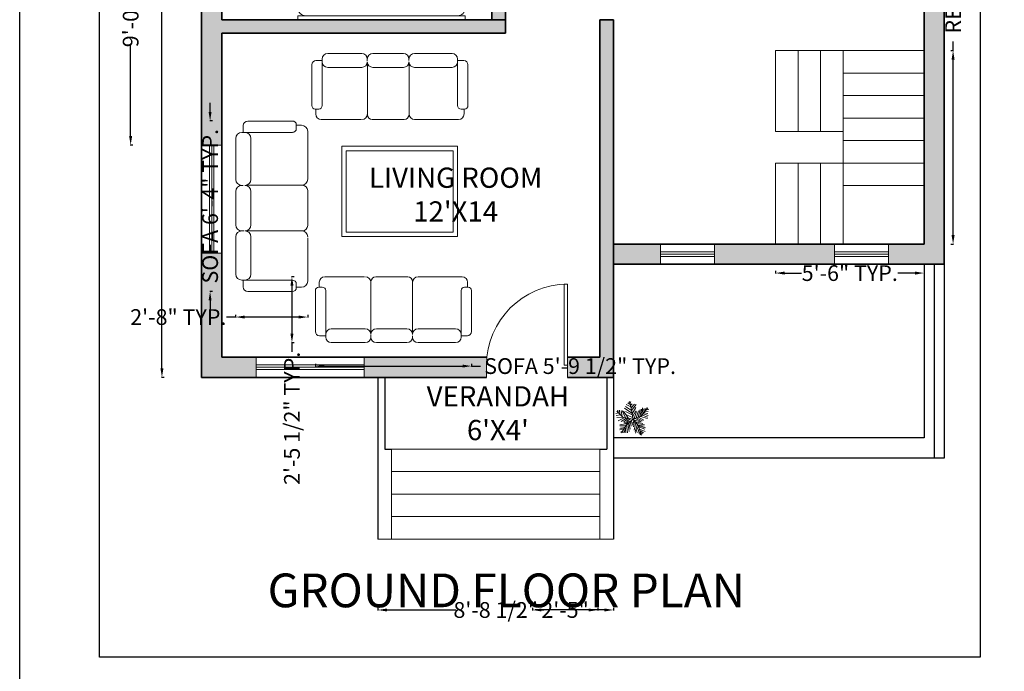
# Model space of a CAD drawing. Units: inches. Extents: x -80 to 1461, y -1239 to 153.
# Tile 2 of 6: x -80 to 358, y -562 to -273. Entities that reach past the tile are written whole.
import ezdxf

# ---------------------------------------------------------------- set-up
doc = ezdxf.new("R2010")
doc.units = ezdxf.units.IN
doc.header["$MEASUREMENT"] = 0
for name, color, linetype, lineweight in [('A-ANNO-DIMS', 2, 'Continuous', 18), ('A-ANNO-TEXT', 7, 'Continuous', 18), ('A-ANNO-TTLB', 7, 'Continuous', 25), ('A-AREA-IDEN', 7, 'Continuous', 18), ('A-FLOR', 7, 'Continuous', 25), ('A-FLOR-STRS', 7, 'Continuous', 20), ('A-FURN', 8, 'Continuous', 18), ('A-GLAZ', 4, 'Continuous', 18), ('A-WALL', 7, 'Continuous', 35), ('A-WALL-PATT', 8, 'Continuous', 13), ('DOOR', 32, 'Continuous', 18), ('TREE', 92, 'Continuous', 13)]:
    doc.layers.add(name, color=color, linetype=linetype, lineweight=lineweight)
doc.styles.get("Standard").update_dxf_attribs({"font": 'arial.ttf'})
doc.dimstyles.get("Standard").update_dxf_attribs({"dimtxt": 7, "dimasz": 4, "dimexe": 0.18, "dimexo": 0.0625, "dimgap": 0.09, "dimtad": 0, "dimdec": 0, "dimzin": 0, "dimdsep": 46, "dimlunit": 3, "dimtxsty": 'Standard', "dimcen": 0.09, "dimadec": 0, "dimazin": 0, "dimtfac": 1, "dimtdec": 0, "dimtofl": 0, "dimtmove": 0, "dimatfit": 3, "dimfxl": 1, "dimfxlon": 1, "dimtolj": 1, "dimtzin": 0, "dimarcsym": 0})

# ---------------------------------------------------------------- blocks, each defined once
blk = doc.blocks.new('*U2')
for p, q in [((0, 0), (0, -6)), ((40, 0), (40, -6))]:
    blk.add_line(p, q)
blk.add_lwpolyline([(0, 0), (0, 40), (1.75, 40), (1.75, 0)], close=True)
blk.add_arc((0, 0), 40, 0, 90)
blk = doc.blocks.new('A$C164346CA')
for p, q in [((0, 2.035), (0, 2)), ((1.5, 2.035), (0, 2.035)), ((1.5, 2), (1.5, 2.035)), ((1.5, 2), (0, 2)), ((0, 1.93), (0, 0.07)), ((0.0919, 1.8624), (0.0919, 1.6069)), ((0.6731, 1.9024), (0.1319, 1.9024)), ((0.7131, 1.6069), (0.7131, 1.8624)), ((0.7828, 1.8624), (0.7828, 1.6069)), ((1.364, 1.9024), (0.8228, 1.9024)), ((1.404, 1.6069), (1.404, 1.8624)), ((1.5, 0.07), (1.5, 1.93)), ((0.1319, 1.5669), (0.6731, 1.5669)), ((0.8228, 1.5669), (1.364, 1.5669)), ((0.8395, 1.4761), (0, 1.4761)), ((0.8395, 1.4761), (1.2448, 1.12)), ((1.5, 1.2611), (0.8395, 1.4761)), ((1.3077, 1.1175), (1.5, 1.2611)), ((0.07, 0), (1.43, 0))]:
    blk.add_line(p, q)
for centre, radius, start, end in [((0.07, 1.93), 0.07, 90, 180), ((1.43, 1.93), 0.07, 0, 90), ((0.1319, 1.8624), 0.04, 90, 180), ((0.6731, 1.8624), 0.04, 0, 90), ((0.8228, 1.8624), 0.04, 90, 180), ((1.364, 1.8624), 0.04, 0, 90), ((0.1319, 1.6069), 0.04, 180, 270), ((0.6731, 1.6069), 0.04, 270, 0), ((0.8228, 1.6069), 0.04, 180, 270), ((1.364, 1.6069), 0.04, 270, 0), ((1.2778, 1.1575), 0.05, 228.69584, 306.75789), ((0.07, 0.07), 0.07, 180, 270), ((1.43, 0.07), 0.07, 270, 0)]:
    blk.add_arc(centre, radius, start, end)
blk = doc.blocks.new('A$C0876780F')
for p, q in [((0.72, 0.95), (0.23, 0.95)), ((1.32, 0.95), (0.88, 0.95)), ((1.48, 0.95), (2.02, 0.95)), ((0, 0.79), (0, 0.21)), ((0.15, 0.85), (0.06, 0.85)), ((0.15, 0.87), (0.15, 0.844)), ((0.15, 0.87), (0.15, 0.85)), ((0.15, 0.21), (0.15, 0.85)), ((0.8, 0.85), (0.8, 0.87)), ((0.8, 0.87), (0.8, 0.85)), ((0.8, 0.87), (0.8, 0.844)), ((0.801, 0.82), (0.801, 0.08)), ((1.4, 0.85), (1.4, 0.87)), ((1.4, 0.85), (1.4, 0.87)), ((1.401, 0.08), (1.401, 0.803)), ((2.1, 0.87), (2.1, 0.85)), ((2.1, 0.87), (2.1, 0.844)), ((2.1, 0.21), (2.1, 0.85)), ((2.1, 0.85), (2.19, 0.85)), ((2.25, 0.79), (2.25, 0.21)), ((0.72, 0.75), (0.23, 0.75)), ((1.32, 0.75), (0.88, 0.75)), ((1.48, 0.75), (2.02, 0.75)), ((0, 0.21), (0, 0.2)), ((0.05, 0.15), (0.1, 0.15)), ((0.056, 0.15), (0.056, 0.08)), ((0.15, 0.2), (0.15, 0.25)), ((2.1, 0.2), (2.1, 0.25)), ((2.2, 0.15), (2.15, 0.15)), ((2.194, 0.15), (2.194, 0.08)), ((2.25, 0.21), (2.25, 0.2)), ((0.136, 0), (0.709, 0)), ((0.801, 0.07), (0.801, 0.08)), ((0.871, 0), (1.331, 0)), ((1.401, 0.07), (1.401, 0.08)), ((2.114, 0), (1.48, 0))]:
    blk.add_line(p, q)
for centre, radius, start, end in [((0.23, 0.87), 0.08, 90, 180), ((0.72, 0.87), 0.08, 0, 90), ((0.88, 0.87), 0.08, 90, 180), ((1.32, 0.87), 0.08, 0, 90), ((1.48, 0.87), 0.08, 90, 180), ((2.02, 0.87), 0.08, 0, 90), ((0.06, 0.79), 0.06, 90, 180), ((0.23, 0.83), 0.08, 180, 270), ((0.23, 0.83), 0.08, 180, 270), ((0.72, 0.83), 0.08, 270, 0), ((0.88, 0.83), 0.08, 180, 270), ((0.88, 0.83), 0.08, 180, 270), ((1.32, 0.83), 0.08, 270, 0), ((1.48, 0.83), 0.08, 180, 270), ((2.02, 0.83), 0.08, 270, 0), ((2.02, 0.83), 0.08, 270, 0), ((2.19, 0.79), 0.06, 0, 90), ((0.05, 0.2), 0.05, 180, 270), ((0.1, 0.2), 0.05, 270, 0), ((0.09, 0.21), 0.06, 350.5377, 0), ((2.16, 0.21), 0.06, 180, 189.4623), ((2.15, 0.2), 0.05, 180, 270), ((2.2, 0.2), 0.05, 270, 0), ((0.136, 0.08), 0.08, 180, 270), ((0.721, 0.08), 0.08, 270, 0), ((0.871, 0.07), 0.07, 180, 270), ((1.331, 0.07), 0.07, 270, 0), ((1.481, 0.08), 0.08, 180, 270), ((2.114, 0.08), 0.08, 270, 0)]:
    blk.add_arc(centre, radius, start, end)
blk = doc.blocks.new('*D12')
at = {"layer": 'A-ANNO-DIMS', "color": 0, "lineweight": -2, "transparency": 16777216}
for p, q in [((-15.61, 30.32), (-16.79, 30.32)), ((-16.61, 26.32), (-16.61, -188.57)), ((-16.61, -427.68), (-16.61, -212.8)), ((-15.61, -431.68), (-16.79, -431.68))]:
    blk.add_line(p, q, dxfattribs=at)
at = {"layer": 'A-ANNO-DIMS', "color": 0, "transparency": 16777216}
for points in [[(-17.27, 26.32), (-15.94, 26.32), (-16.61, 30.32)], [(-17.27, -427.68), (-15.94, -427.68), (-16.61, -431.68)]]:
    blk.add_solid(points, dxfattribs=at)
at = {"layer": 'Defpoints', "color": 0, "transparency": 16777216}
for p in [(0.99, 30.32), (-16.61, -431.68), (0.99, -431.68)]:
    blk.add_point(p, dxfattribs=at)
at = {"layer": 'A-ANNO-DIMS', "color": 0, "transparency": 16777216, "insert": (-16.61, -200.68), "char_height": 7, "attachment_point": 5, "rotation": 90}
blk.add_mtext('\\A1;38\'-6"', dxfattribs=at)
blk = doc.blocks.new('*U10')
for p, q in [((-3.665, 19.273), (-27.574, 35.527)), ((-5.114, 28.097), (-24.676, 40.636)), ((-7.288, 39.707), (-21.778, 46.673)), ((-8.737, 47.138), (-17.069, 52.711)), ((-10.186, 53.64), (-13.084, 55.962)), ((0, 0), (-10.5, 57)), ((-9.099, 51.782), (-6.563, 55.962)), ((-7.65, 43.423), (-2.578, 49.46)), ((-5.839, 35.992), (4.667, 48.067)), ((-5.114, 27.632), (10.463, 46.673)), ((-2.941, 16.486), (8.652, 37.85)), ((22.055, 7.198), (27.489, 32.277)), ((27, 9), (48, 36)), ((27.127, 9.056), (31.112, 35.992)), ((35.096, 32.741), (37.27, 22.524)), ((38.719, 34.134), (41.979, 28.561)), ((44.153, 36.456), (45.239, 32.741)), ((-47.498, 19.737), (-55.83, 18.344)), ((-40.615, 13.7), (-55.105, 10.913)), ((-31.5, 4.5), (-52.5, 25.5)), ((-33.37, 6.269), (-52.207, 5.34)), ((-48.585, 21.131), (-49.309, 29.026)), ((-28.299, 3.483), (-47.86, -5.805)), ((-43.513, 28.561), (-42.427, 15.558)), ((-38.442, 26.239), (-34.819, 7.663)), ((-21.416, 3.018), (-38.079, -8.128)), ((-35.544, 28.097), (-24.314, 3.947)), ((0, 0), (-31.5, 4.5)), ((-14.533, 2.09), (-30.834, 25.31)), ((-15.982, 2.09), (-30.11, -9.521)), ((-24.314, 23.917), (-2.941, 13.7)), ((0, 0), (-22.5, -19.5)), ((-6.563, 1.161), (-21.416, -8.128)), ((-20.691, 13.7), (-1.129, 4.876)), ((-1.129, 6.734), (9.014, 26.704)), ((0, 0), (27, 9)), ((0, 0), (18, -22.5)), ((3.942, 1.625), (11.187, 24.381)), ((6.478, 1.625), (26.04, -8.592)), ((10.101, 3.483), (17.708, 26.239)), ((11.187, 3.483), (30.749, -5.805)), ((16.259, 5.805), (23.142, 31.348)), ((18.07, 5.805), (35.096, -3.483)), ((24.229, 7.663), (46.688, 1.625)), ((29.662, 12.307), (48.137, 6.269)), ((31.836, 30.883), (32.561, 16.486)), ((33.285, 16.486), (48.862, 10.913)), ((36.183, 19.737), (48.137, 17.88)), ((40.53, 25.775), (48.862, 24.846)), ((43.791, 29.954), (51.036, 30.883)), ((-17.431, -15.094), (-42.789, -18.809)), ((-28.299, -29.026), (-42.789, -31.348)), ((-24.314, -21.596), (-42.427, -22.06)), ((-26.849, -26.24), (-40.253, -25.775)), ((-22.5, -19.5), (-37.5, -45)), ((-15.257, -12.772), (-30.11, -12.772)), ((-29.023, -30.884), (-27.936, -43.887)), ((-25.038, -23.918), (-22.865, -45.281)), ((-20.691, -18.345), (-17.793, -44.352)), ((-6.563, -5.805), (-19.967, -9.985)), ((-17.069, -15.094), (-12.721, -40.172)), ((-13.446, -11.378), (-8.737, -32.741)), ((-9.461, -8.592), (-6.201, -23.453)), ((-4.752, -3.483), (-3.665, -14.629)), ((2.493, -3.019), (-1.491, -20.202)), ((1.769, -2.555), (24.229, -9.521)), ((5.029, -6.27), (2.131, -25.775)), ((9.014, -11.378), (3.58, -35.992)), ((14.085, -16.951), (6.478, -40.172)), ((7.565, -9.056), (32.198, -14.629)), ((18.07, -22.524), (8.289, -45.745)), ((12.274, -15.094), (36.907, -18.809)), ((20.244, -30.419), (15.897, -44.816)), ((16.259, -19.738), (36.183, -22.989)), ((18, -22.5), (27, -52.5)), ((18.433, -22.524), (40.53, -29.026)), ((19.157, -25.311), (38.719, -33.206)), ((-30.834, -34.135), (-42.427, -35.528)), ((-34.457, -39.708), (-40.978, -42.494)), ((-32.646, -36.921), (-31.921, -44.352)), ((22.78, -37.85), (19.519, -48.532)), ((21.331, -32.741), (39.081, -40.636)), ((22.78, -38.314), (34.372, -44.816)), ((24.591, -45.745), (23.142, -50.854)), ((24.591, -43.423), (30.749, -47.603)), ((26.764, -49.925), (28.213, -50.854))]:
    blk.add_line(p, q)
blk = doc.blocks.new('WIN-48IN')
for p, q in [((0, 9), (0, 0)), ((48, 9), (0, 9)), ((48, 0), (48, 9)), ((0, 5.5), (48, 5.5)), ((0, 4.5), (48, 4.5)), ((0, 3.5), (48, 3.5)), ((0, 0), (36, 0)), ((36, 0), (48, 0))]:
    blk.add_line(p, q)
blk = doc.blocks.new('WIN-24IN')
for p, q in [((0, 9), (0, 0)), ((0, 9), (24, 9)), ((24, 9), (24, 0)), ((0, 5.5), (24, 5.5)), ((0, 4.5), (24, 4.5)), ((0, 3.5), (24, 3.5)), ((0, 0), (24, 0))]:
    blk.add_line(p, q)
blk = doc.blocks.new('COFFEE-TABLE')
for points in [[(0, 40.15), (51.49, 40.15), (51.49, 0), (0, 0)], [(2, 38.15), (49.49, 38.15), (49.49, 2), (2, 2)]]:
    blk.add_lwpolyline(points, close=True)
blk = doc.blocks.new('STAIR-RETURN-PLAN')
for p, q in [((0, 86), (0, 50)), ((0, 86), (30, 86)), ((10, 86), (10, 50)), ((20, 86), (20, 50)), ((66, 86), (30, 86)), ((30, 86), (30, 50)), ((66, 76), (30, 76)), ((66, 66), (30, 66)), ((66, 56), (30, 56)), ((0, 50), (30, 50)), ((30, 50), (30, 36)), ((66, 46), (30, 46)), ((0, 36), (0, 0)), ((0, 36), (30, 36)), ((10, 36), (10, 0)), ((20, 36), (20, 0)), ((66, 36), (30, 36)), ((30, 36), (30, 0)), ((66, 26), (30, 26))]:
    blk.add_line(p, q)
blk = doc.blocks.new('*D42')
at = {"layer": 'A-ANNO-DIMS', "color": 0, "lineweight": -2, "transparency": 16777216}
for p, q in [((4.78, -313.72), (4.78, -309.72)), ((5.78, -317.72), (4.6, -317.72)), ((5.78, -393.5), (4.6, -393.5)), ((4.78, -397.5), (4.78, -401.5))]:
    blk.add_line(p, q, dxfattribs=at)
at = {"layer": 'A-ANNO-DIMS', "color": 0, "transparency": 16777216}
for points in [[(4.11, -313.72), (5.44, -313.72), (4.78, -317.72)], [(4.11, -397.5), (5.44, -397.5), (4.78, -393.5)]]:
    blk.add_solid(points, dxfattribs=at)
at = {"layer": 'Defpoints', "color": 0, "transparency": 16777216}
for p in [(4.78, -317.72), (16.14, -317.72), (16.14, -393.5)]:
    blk.add_point(p, dxfattribs=at)
at = {"layer": 'A-ANNO-DIMS', "color": 0, "transparency": 16777216, "insert": (4.78, -355.61), "char_height": 7, "attachment_point": 5, "rotation": 90}
blk.add_mtext('\\A1;SOFA 6\'-4" TYP.', dxfattribs=at)
blk = doc.blocks.new('*D43')
at = {"layer": 'A-ANNO-DIMS', "color": 0, "lineweight": -2, "transparency": 16777216}
for p, q in [((16.14, -404.87), (12.14, -404.87)), ((16.14, -403.87), (16.14, -405.05)), ((44.14, -404.87), (20.14, -404.87)), ((48.14, -403.87), (48.14, -405.05))]:
    blk.add_line(p, q, dxfattribs=at)
at = {"layer": 'A-ANNO-DIMS', "color": 0, "transparency": 16777216}
for points in [[(20.14, -404.2), (20.14, -405.53), (16.14, -404.87)], [(44.14, -404.2), (44.14, -405.53), (48.14, -404.87)]]:
    blk.add_solid(points, dxfattribs=at)
at = {"layer": 'Defpoints', "color": 0, "transparency": 16777216}
for p in [(16.14, -393.5), (48.14, -393.5), (16.14, -404.87)]:
    blk.add_point(p, dxfattribs=at)
at = {"layer": 'A-ANNO-DIMS', "color": 0, "transparency": 16777216, "insert": (-9.34, -404.87), "char_height": 7, "attachment_point": 5}
blk.add_mtext('\\A1;2\'-8" TYP.', dxfattribs=at)
blk = doc.blocks.new('*D44')
at = {"layer": 'A-ANNO-DIMS', "color": 0, "lineweight": -2, "transparency": 16777216}
for p, q in [((51.55, -425.67), (51.55, -426.85)), ((55.55, -426.67), (116.93, -426.67)), ((120.93, -425.67), (120.93, -426.85)), ((120.93, -426.67), (124.93, -426.67))]:
    blk.add_line(p, q, dxfattribs=at)
at = {"layer": 'A-ANNO-DIMS', "color": 0, "transparency": 16777216}
for points in [[(55.55, -426), (55.55, -427.33), (51.55, -426.67)], [(116.93, -426), (116.93, -427.33), (120.93, -426.67)]]:
    blk.add_solid(points, dxfattribs=at)
at = {"layer": 'Defpoints', "color": 0, "transparency": 16777216}
for p in [(51.55, -416.26), (120.93, -416.26), (120.93, -426.67)]:
    blk.add_point(p, dxfattribs=at)
at = {"layer": 'A-ANNO-DIMS', "color": 0, "transparency": 16777216, "insert": (169.17, -426.67), "char_height": 7, "attachment_point": 5}
blk.add_mtext('\\A1;SOFA 5\'-9 1/2" TYP.', dxfattribs=at)
blk = doc.blocks.new('*D45')
at = {"layer": 'A-ANNO-DIMS', "color": 0, "lineweight": -2, "transparency": 16777216}
for p, q in [((42.14, -386.96), (40.96, -386.96)), ((41.14, -390.96), (41.14, -412.26)), ((42.14, -416.26), (40.96, -416.26)), ((41.14, -416.26), (41.14, -420.26))]:
    blk.add_line(p, q, dxfattribs=at)
at = {"layer": 'A-ANNO-DIMS', "color": 0, "transparency": 16777216}
for points in [[(40.48, -390.96), (41.81, -390.96), (41.14, -386.96)], [(40.48, -412.26), (41.81, -412.26), (41.14, -416.26)]]:
    blk.add_solid(points, dxfattribs=at)
at = {"layer": 'Defpoints', "color": 0, "transparency": 16777216}
for p in [(51.55, -386.96), (41.14, -416.26), (51.55, -416.26)]:
    blk.add_point(p, dxfattribs=at)
at = {"layer": 'A-ANNO-DIMS', "color": 0, "transparency": 16777216, "insert": (41.14, -449.9), "char_height": 7, "attachment_point": 5, "rotation": 90}
blk.add_mtext('\\A1;2\'-5 1/2" TYP.', dxfattribs=at)
blk = doc.blocks.new('*D56')
at = {"layer": 'A-ANNO-DIMS', "color": 0, "lineweight": -2, "transparency": 16777216}
for p, q in [((334.89, -286.42), (334.89, -282.42)), ((333.89, -286.42), (335.07, -286.42)), ((334.89, -368.42), (334.89, -290.42)), ((333.89, -372.42), (335.07, -372.42))]:
    blk.add_line(p, q, dxfattribs=at)
at = {"layer": 'A-ANNO-DIMS', "color": 0, "transparency": 16777216}
for points in [[(334.22, -290.42), (335.56, -290.42), (334.89, -286.42)], [(334.22, -368.42), (335.56, -368.42), (334.89, -372.42)]]:
    blk.add_solid(points, dxfattribs=at)
at = {"layer": 'Defpoints', "color": 0, "transparency": 16777216}
for p in [(321.99, -286.42), (334.89, -286.42), (321.99, -372.42)]:
    blk.add_point(p, dxfattribs=at)
at = {"layer": 'A-ANNO-DIMS', "color": 0, "transparency": 16777216, "insert": (334.89, -223.69), "char_height": 7, "attachment_point": 5, "rotation": 90}
blk.add_mtext('\\A1;RETURN STAIR 7\'-2" TYP.', dxfattribs=at)
blk = doc.blocks.new('*D57')
at = {"layer": 'A-ANNO-DIMS', "color": 0, "lineweight": -2, "transparency": 16777216}
for p, q in [((255.99, -384.32), (255.99, -385.5)), ((321.99, -384.32), (321.99, -385.5)), ((259.99, -385.32), (267.57, -385.32)), ((317.99, -385.32), (310.41, -385.32))]:
    blk.add_line(p, q, dxfattribs=at)
at = {"layer": 'A-ANNO-DIMS', "color": 0, "transparency": 16777216}
for points in [[(259.99, -384.66), (259.99, -385.99), (255.99, -385.32)], [(317.99, -384.66), (317.99, -385.99), (321.99, -385.32)]]:
    blk.add_solid(points, dxfattribs=at)
at = {"layer": 'Defpoints', "color": 0, "transparency": 16777216}
for p in [(255.99, -372.42), (321.99, -372.42), (321.99, -385.32)]:
    blk.add_point(p, dxfattribs=at)
at = {"layer": 'A-ANNO-DIMS', "color": 0, "transparency": 16777216, "insert": (288.99, -385.32), "char_height": 7, "attachment_point": 5}
blk.add_mtext('\\A1;5\'-6" TYP.', dxfattribs=at)
blk = doc.blocks.new('*D72')
at = {"layer": 'A-ANNO-DIMS', "color": 0, "lineweight": -2, "transparency": 16777216}
for p, q in [((412.49, 30.32), (413.67, 30.32)), ((413.49, 26.32), (413.49, -224.38)), ((413.49, -499.58), (413.49, -248.89)), ((412.49, -503.58), (413.67, -503.58))]:
    blk.add_line(p, q, dxfattribs=at)
at = {"layer": 'A-ANNO-DIMS', "color": 0, "transparency": 16777216}
for points in [[(412.82, 26.32), (414.16, 26.32), (413.49, 30.32)], [(412.82, -499.58), (414.16, -499.58), (413.49, -503.58)]]:
    blk.add_solid(points, dxfattribs=at)
at = {"layer": 'Defpoints', "color": 0, "transparency": 16777216}
for p in [(330.99, 30.32), (183.99, -503.58), (413.49, -503.58)]:
    blk.add_point(p, dxfattribs=at)
at = {"layer": 'A-ANNO-DIMS', "color": 0, "transparency": 16777216, "insert": (413.49, -236.63), "char_height": 7, "attachment_point": 5, "rotation": 90}
blk.add_mtext('\\A1;44\'-6"', dxfattribs=at)
blk = doc.blocks.new('*D74')
at = {"layer": 'A-ANNO-DIMS', "color": 0, "lineweight": -2, "transparency": 16777216}
for p, q in [((127.63, 111.82), (127.63, 113)), ((131.63, 112.82), (136.23, 112.82)), ((159.62, 112.82), (155.02, 112.82)), ((163.62, 111.82), (163.62, 113))]:
    blk.add_line(p, q, dxfattribs=at)
at = {"layer": 'A-ANNO-DIMS', "color": 0, "transparency": 16777216}
for points in [[(131.63, 113.48), (131.63, 112.15), (127.63, 112.82)], [(159.62, 113.48), (159.62, 112.15), (163.62, 112.82)]]:
    blk.add_solid(points, dxfattribs=at)
at = {"layer": 'Defpoints', "color": 0, "transparency": 16777216}
for p in [(163.62, 112.82), (127.63, -431.68), (163.62, -431.68)]:
    blk.add_point(p, dxfattribs=at)
at = {"layer": 'A-ANNO-DIMS', "color": 0, "transparency": 16777216, "insert": (145.63, 112.82), "char_height": 7, "attachment_point": 5}
blk.add_mtext('\\A1;3\'-0"', dxfattribs=at)
blk = doc.blocks.new('*D75')
at = {"layer": 'A-ANNO-DIMS', "color": 0, "lineweight": -2, "transparency": 16777216}
for p, q in [((79.36, -534.08), (79.36, -535.26)), ((83.36, -535.08), (114.12, -535.08)), ((179.99, -535.08), (149.23, -535.08)), ((183.99, -534.08), (183.99, -535.26))]:
    blk.add_line(p, q, dxfattribs=at)
at = {"layer": 'A-ANNO-DIMS', "color": 0, "transparency": 16777216}
for points in [[(83.36, -534.42), (83.36, -535.75), (79.36, -535.08)], [(179.99, -534.42), (179.99, -535.75), (183.99, -535.08)]]:
    blk.add_solid(points, dxfattribs=at)
at = {"layer": 'Defpoints', "color": 0, "transparency": 16777216}
for p in [(79.36, -503.58), (183.99, -503.58), (183.99, -535.08)]:
    blk.add_point(p, dxfattribs=at)
at = {"layer": 'A-ANNO-DIMS', "color": 0, "transparency": 16777216, "insert": (131.68, -535.08), "char_height": 7, "attachment_point": 5}
blk.add_mtext('\\A1;8\'-8 1/2"', dxfattribs=at)
blk = doc.blocks.new('*D76')
at = {"layer": 'A-ANNO-DIMS', "color": 0, "lineweight": -2, "transparency": 16777216}
for p, q in [((147.99, -534.08), (147.99, -535.26)), ((151.99, -535.08), (153.04, -535.08)), ((172.99, -535.08), (171.94, -535.08)), ((176.99, -534.08), (176.99, -535.26))]:
    blk.add_line(p, q, dxfattribs=at)
at = {"layer": 'A-ANNO-DIMS', "color": 0, "transparency": 16777216}
for points in [[(151.99, -534.42), (151.99, -535.75), (147.99, -535.08)], [(172.99, -534.42), (172.99, -535.75), (176.99, -535.08)]]:
    blk.add_solid(points, dxfattribs=at)
at = {"layer": 'Defpoints', "color": 0, "transparency": 16777216}
for p in [(147.99, -68.68), (176.99, -68.68), (176.99, -535.08)]:
    blk.add_point(p, dxfattribs=at)
at = {"layer": 'A-ANNO-DIMS', "color": 0, "transparency": 16777216, "insert": (162.49, -535.08), "char_height": 7, "attachment_point": 5}
blk.add_mtext('\\A1;2\'-5"', dxfattribs=at)
blk = doc.blocks.new('*D83')
at = {"layer": 'A-ANNO-DIMS', "color": 0, "lineweight": -2, "transparency": 16777216}
for p, q in [((-29.51, -220.33), (-30.69, -220.33)), ((-30.51, -224.33), (-30.51, -265)), ((-30.51, -324.45), (-30.51, -283.78)), ((-29.51, -328.45), (-30.69, -328.45))]:
    blk.add_line(p, q, dxfattribs=at)
at = {"layer": 'A-ANNO-DIMS', "color": 0, "transparency": 16777216}
for points in [[(-31.18, -224.33), (-29.84, -224.33), (-30.51, -220.33)], [(-31.18, -324.45), (-29.84, -324.45), (-30.51, -328.45)]]:
    blk.add_solid(points, dxfattribs=at)
at = {"layer": 'Defpoints', "color": 0, "transparency": 16777216}
for p in [(0.99, -220.33), (-30.51, -328.45), (0.99, -328.45)]:
    blk.add_point(p, dxfattribs=at)
at = {"layer": 'A-ANNO-DIMS', "color": 0, "transparency": 16777216, "insert": (-30.51, -274.39), "char_height": 7, "attachment_point": 5, "rotation": 90}
blk.add_mtext('\\A1;9\'-0"', dxfattribs=at)

msp = doc.modelspace()

# ---------------------------------------------------------------- hatches: boundary and pattern name
at = {"layer": 'A-WALL-PATT'}
h = msp.add_hatch(color=256, dxfattribs=at)
h.dxf.hatch_style = 1
h.paths.add_polyline_path([(162.37, 30.32), (98.86, 30.32), (98.86, 21.32), (141.99, 21.32), (141.99, -81.2, -0.004167), (142.59, -81.2), (147.99, -81.2), (147.99, 21.32), (162.37, 21.32)])
h.paths.add_polyline_path([(330.99, 30.32), (297.57, 30.32), (297.57, 21.32), (321.99, 21.32), (321.99, -3.69), (330.99, -3.69)])
h.paths.add_polyline_path([(249.57, 30.32), (186.37, 30.32), (186.37, 21.32), (192.39, 21.32), (207.99, 21.32), (207.99, -104.68), (213.99, -104.68), (213.99, -99.28), (213.99, -63.28), (213.99, 21.32), (249.57, 21.32)])
h.paths.add_polyline_path([(330.99, -39.69), (321.99, -39.69), (321.99, -98.68), (249.99, -98.68, -0.004167), (249.99, -99.28), (249.99, -104.68), (321.99, -104.68), (321.99, -132.06), (330.99, -132.06)])
h.paths.add_polyline_path([(330.99, -156.06), (321.99, -156.06), (321.99, -166.56), (321.99, -188.68), (261.99, -188.68), (261.99, -133.64, -0.014233), (260.34, -133.68), (255.99, -133.68), (255.99, -194.68), (321.99, -194.68), (321.99, -372.42), (306.16, -372.42), (306.16, -381.42), (330.99, -381.42)])
h = msp.add_hatch(color=256, dxfattribs=at)
h.dxf.hatch_style = 1
h.paths.add_polyline_path([(183.99, -272.68), (177.99, -272.68), (177.99, -422.68), (163.62, -422.68), (163.62, -426.28), (163.62, -431.68), (183.99, -431.68)])
h.paths.add_polyline_path([(9.99, -220.33), (0.99, -220.33), (0.99, -328.45), (9.99, -328.45), (9.99, -278.68), (135.99, -278.68), (135.99, -272.68), (9.99, -272.68)])
h.paths.add_polyline_path([(135.99, -164.68), (130.59, -164.68, -0.004167), (129.99, -164.68), (129.99, -272.68), (135.99, -272.68)])
h.paths.add_polyline_path([(127.62, -426.28, -0.025047), (127.8, -422.68), (73.28, -422.68), (73.28, -431.68), (127.62, -431.68)])
h.paths.add_polyline_path([(25.28, -422.68), (9.99, -422.68), (9.99, -376.45), (0.99, -376.45), (0.99, -431.68), (25.28, -431.68)])
h = msp.add_hatch(color=256, dxfattribs=at)
h.dxf.hatch_style = 1
h.paths.add_polyline_path([(282.16, -372.42), (228.94, -372.42), (228.94, -381.42), (282.16, -381.42)])
h.paths.add_polyline_path([(204.94, -372.42), (183.99, -372.42), (183.99, -381.42), (204.94, -381.42)])

# ---------------------------------------------------------------- linework, layer by layer
at = {"layer": 'A-ANNO-TTLB'}
for points in [[(-79.81, 141.36), (1461.09, 141.36), (1461.09, -1239.28), (-79.81, -1239.28)], [(-44.36, 71.88), (346.97, 71.88), (346.97, -556.04), (-44.36, -556.04)]]:
    msp.add_lwpolyline(points, close=True, dxfattribs=at)
at = {"layer": 'A-FLOR'}
for p, q in [((321.99, -381.42), (321.99, -458.56)), ((326.49, -381.42), (326.49, -467.56)), ((330.99, -381.42), (330.99, -467.56)), ((79.36, -431.68), (79.36, -503.58)), ((82.36, -431.68), (82.36, -463.58)), ((180.99, -431.68), (180.99, -463.58)), ((183.99, -431.68), (183.99, -503.58)), ((321.99, -458.56), (183.99, -458.56)), ((82.36, -463.58), (85.36, -463.58)), ((177.99, -463.58), (180.99, -463.58)), ((330.99, -467.56), (183.99, -467.56))]:
    msp.add_line(p, q, dxfattribs=at)
at = {"layer": 'A-FLOR-STRS'}
for p, q in [((85.36, -463.58), (85.36, -503.58)), ((177.99, -463.58), (85.36, -463.58)), ((177.99, -463.58), (177.99, -503.58)), ((177.99, -473.58), (85.36, -473.58)), ((177.99, -483.58), (85.36, -483.58)), ((177.99, -493.58), (85.36, -493.58)), ((183.99, -503.58), (79.36, -503.58))]:
    msp.add_line(p, q, dxfattribs=at)
at = {"layer": 'A-WALL'}
for p, q in [((0.99, 30.32), (0.99, -431.68)), ((330.99, 30.32), (330.99, -381.42)), ((9.99, -128.68), (9.99, -272.68)), ((129.99, -164.68), (129.99, -272.68)), ((135.99, -164.68), (135.99, -278.68)), ((321.99, -194.68), (321.99, -372.42)), ((9.99, -272.68), (135.99, -272.68)), ((177.99, -272.68), (177.99, -422.68)), ((177.99, -272.68), (183.99, -272.68)), ((183.99, -272.68), (183.99, -431.68)), ((9.99, -278.68), (135.99, -278.68)), ((9.99, -278.68), (9.99, -422.68)), ((183.99, -372.42), (321.99, -372.42)), ((183.99, -381.42), (330.99, -381.42)), ((9.99, -422.68), (127.8, -422.68)), ((163.62, -422.68), (177.99, -422.68)), ((0.99, -431.68), (127.63, -431.68)), ((163.62, -431.68), (183.99, -431.68))]:
    msp.add_line(p, q, dxfattribs=at)

# ---------------------------------------------------------------- block references
at = {"layer": 'A-FLOR-STRS'}
msp.add_blockref('STAIR-RETURN-PLAN', (255.99, -372.42), dxfattribs=at)
at = {"layer": 'A-FURN'}
for name, p, xscale, yscale, zscale, rotation in [('A$C164346CA', (118.17, -171.81), 49.56739756478314, 49.56739756478314, 49.56739756478314, 180), ('A$C0876780F', (48.14, -393.5), 33.67837588954761, 33.67837588954761, 33.67837588954761, 90), ('A$C0876780F', (51.55, -386.96), -30.83775321962601, 30.83775321962601, 30.83775321962601, 180)]:
    msp.add_blockref(name, p, dxfattribs=dict(at, xscale=xscale, yscale=yscale, zscale=zscale, rotation=rotation))
at = {"layer": 'A-FURN', "xscale": 30.83775321962601, "yscale": 30.83775321962601, "zscale": 30.83775321962601}
msp.add_blockref('A$C0876780F', (49.97, -317.03), dxfattribs=at)
at = {"layer": 'A-FURN'}
msp.add_blockref('COFFEE-TABLE', (63.24, -369.09), dxfattribs=at)
at = {"layer": 'A-GLAZ', "rotation": 89.99999999999996}
msp.add_blockref('WIN-48IN', (9.99, -376.45), dxfattribs=at)
at = {"layer": 'A-GLAZ'}
for name, p in [('WIN-24IN', (204.94, -381.42)), ('WIN-24IN', (282.16, -381.42)), ('WIN-48IN', (25.28, -431.68))]:
    msp.add_blockref(name, p, dxfattribs=at)
at = {"layer": 'DOOR', "xscale": -0.9, "yscale": 0.9, "zscale": 0.9}
msp.add_blockref('*U2', (163.62, -426.28), dxfattribs=at)
at = {"layer": 'TREE', "xscale": 0.1370045651508197, "yscale": 0.1370045651508197, "zscale": 0.1370045651508197}
msp.add_blockref('*U10', (192.68, -450.19), dxfattribs=at)

# ---------------------------------------------------------------- texts
at = {"layer": 'A-ANNO-TEXT', "insert": (13.9, -518.87), "char_height": 15, "attachment_point": 1}
msp.add_mtext_dynamic_manual_height_columns('\\pxqc;GROUND FLOOR PLAN', width=245.0183, gutter_width=1, heights=[0], dxfattribs=at)
at = {"layer": 'A-AREA-IDEN', "char_height": 9, "attachment_point": 1}
for s, insert in [("\\pxqc;LIVING ROOM\\P12'X14", (65.52, -338.43)), ("\\pxqc;VERANDAH\\P6'X4'", (84.27, -435.6))]:
    msp.add_mtext_dynamic_manual_height_columns(s, width=96.7224, gutter_width=1, heights=[0], dxfattribs=dict(at, insert=insert))

# ---------------------------------------------------------------- dimensions: what is measured, and where the dimension line sits
at = {"layer": 'A-ANNO-DIMS'}
for base, p1, p2, picture, middle in [((163.62, 112.82), (127.63, -431.68), (163.62, -431.68), '*D74', (145.63, 112.82)), ((176.99, -535.08), (147.99, -68.68), (176.99, -68.68), '*D76', (162.49, -535.08)), ((183.99, -535.08), (79.36, -503.58), (183.99, -503.58), '*D75', (131.68, -535.08))]:
    dim = msp.add_linear_dim(base=base, p1=p1, p2=p2, dimstyle='Standard', override={"dimdec": 1, "dimlfac": 1, "dimrnd": 0, "dimzin": 1, "dimdsep": 46, "dimlunit": 4, "dimfrac": 2}, dxfattribs=at)
    dim.commit()
    dim.dimension.update_dxf_attribs({"geometry": picture, "text_midpoint": middle})
for base, p1, p2, override, picture, middle in [((-16.61, -431.68), (0.99, 30.32), (0.99, -431.68), {"dimclrd": 0, "dimclre": 0, "dimclrt": 0}, '*D12', (-16.61, -200.68)), ((413.49, -503.58), (330.99, 30.32), (183.99, -503.58), {"dimdec": 1, "dimlfac": 1, "dimrnd": 0, "dimzin": 1, "dimdsep": 46, "dimlunit": 4, "dimfrac": 2}, '*D72', (413.49, -236.63)), ((-30.51, -328.45), (0.99, -220.33), (0.99, -328.45), {"dimdec": 1, "dimlfac": 1, "dimrnd": 0, "dimzin": 1, "dimdsep": 46, "dimlunit": 4, "dimfrac": 2}, '*D83', (-30.51, -274.39))]:
    dim = msp.add_linear_dim(base=base, p1=p1, p2=p2, angle=90, dimstyle='Standard', override=override, dxfattribs=at)
    dim.commit()
    dim.dimension.update_dxf_attribs({"geometry": picture, "text_midpoint": middle})
for base, p1, p2, angle, text, picture, middle in [((334.89, -286.42), (321.99, -372.42), (321.99, -286.42), 90, 'RETURN STAIR <> TYP.', '*D56', (334.89, -223.69)), ((4.78, -317.72), (16.14, -393.5), (16.14, -317.72), 90, 'SOFA <> TYP.', '*D42', (4.78, -355.61)), ((41.14, -416.26), (51.55, -386.96), (51.55, -416.26), 270, '<> TYP.', '*D45', (41.14, -449.9)), ((16.14, -404.87), (48.14, -393.5), (16.14, -393.5), 180, '<> TYP.', '*D43', (-9.34, -404.87))]:
    dim = msp.add_linear_dim(base=base, p1=p1, p2=p2, angle=angle, text=text, dimstyle='Standard', override={"dimdec": 1, "dimlfac": 1, "dimrnd": 0, "dimzin": 1, "dimdsep": 46, "dimlunit": 4, "dimfrac": 2}, dxfattribs=at)
    dim.commit()
    dim.dimension.update_dxf_attribs({"geometry": picture, "text_midpoint": middle})
for base, p1, p2, text, picture, middle in [((321.99, -385.32), (255.99, -372.42), (321.99, -372.42), '<> TYP.', '*D57', (288.99, -385.32)), ((120.93, -426.67), (51.55, -416.26), (120.93, -416.26), 'SOFA <> TYP.', '*D44', (169.17, -426.67))]:
    dim = msp.add_linear_dim(base=base, p1=p1, p2=p2, text=text, dimstyle='Standard', override={"dimdec": 1, "dimlfac": 1, "dimrnd": 0, "dimzin": 1, "dimdsep": 46, "dimlunit": 4, "dimfrac": 2}, dxfattribs=at)
    dim.commit()
    dim.dimension.update_dxf_attribs({"geometry": picture, "text_midpoint": middle})

doc.saveas('drawing.dxf')
